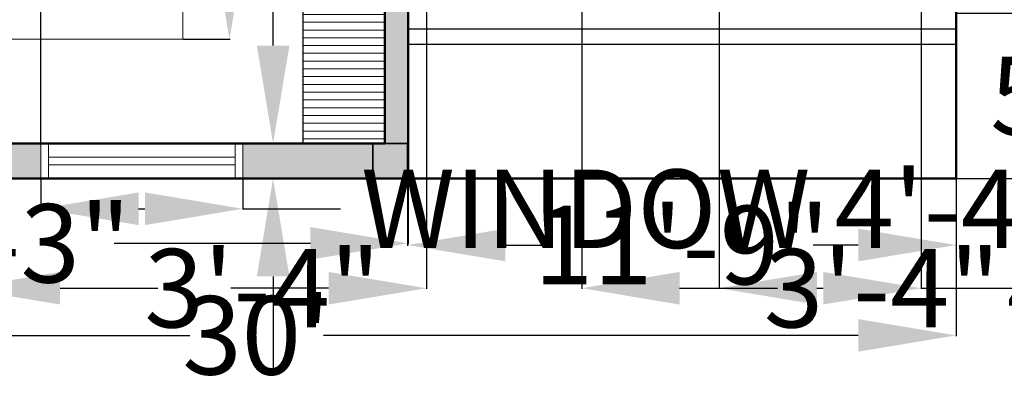
# Model space of a CAD drawing. Units: inches. Extents: x 25 to 82118, y 10 to 6494.
# Tile 3 of 9: x 40833 to 41087, y 3093 to 3189. Entities that reach past the tile are written whole.
import ezdxf

# ---------------------------------------------------------------- set-up
doc = ezdxf.new("R2010")
doc.units = ezdxf.units.IN
doc.header["$MEASUREMENT"] = 0
for name, color, linetype, lineweight in [('A-ANNO-DIMS', 2, 'Continuous', 18), ('A-FLOR-CASE', 8, 'Continuous', 25), ('A-FLOR-CASE-PATT', 9, 'Continuous', 13), ('A-FLOR-STRS', 7, 'Continuous', 25), ('A-FURN', 8, 'Continuous', 18), ('A-GLAZ', 4, 'Continuous', 18), ('A-WALL', 7, 'Continuous', 50)]:
    doc.layers.add(name, color=color, linetype=linetype, lineweight=lineweight)
doc.layers.add('A-COLS', color=30, linetype='Continuous', lineweight=35, true_color=0xf26722)
doc.layers.add('A-WALL-PATT', color=18, linetype='Continuous', lineweight=13, true_color=0x000000)
doc.styles.get("Standard").update_dxf_attribs({"font": 'arial.ttf'})
doc.dimstyles.get("Standard").update_dxf_attribs({"dimtxt": 20.18, "dimasz": 25.18, "dimexe": 0.18, "dimexo": 0.0625, "dimgap": 0.09, "dimtad": 0, "dimtih": 1, "dimtoh": 1, "dimdec": 0, "dimzin": 0, "dimdsep": 46, "dimlunit": 3, "dimtxsty": 'Standard', "dimcen": 0.09, "dimadec": 0, "dimazin": 0, "dimtfac": 1, "dimtdec": 0, "dimtofl": 0, "dimtmove": 0, "dimatfit": 3, "dimfxl": 1, "dimtolj": 1, "dimtzin": 0, "dimarcsym": 0})

# ---------------------------------------------------------------- blocks, each defined once
blk = doc.blocks.new('Bed - Queen')
for p, q in [((0, -80.00003), (0, 0)), ((0, 0), (59.99999, 0)), ((59.99999, 0), (59.99999, -80.00003)), ((7.99999, -1.2), (28.79998, -1.2)), ((7.99999, -14.4), (7.99999, -1.2)), ((28.79998, -1.2), (28.79998, -14.4)), ((31.19999, -1.2), (51.99999, -1.2)), ((31.19999, -14.4), (31.19999, -1.2)), ((51.99999, -1.2), (51.99999, -16.4)), ((0, -14.4), (44.8, -14.4)), ((59.99999, -29.6), (44.8, -14.4)), ((44.8, -14.4), (44.8, -29.6)), ((44.8, -16.8), (0, -16.8)), ((51.99999, -16.4), (46.79936, -16.4)), ((44.8, -29.6), (59.99999, -29.6)), ((59.99999, -80.00003), (0, -80.00003))]:
    blk.add_line(p, q)
blk = doc.blocks.new('*D16')
at = {"layer": 'A-ANNO-DIMS', "color": 0, "lineweight": -2, "transparency": 16777216}
for p, q in [((41074.33, 3531.88), (41191.01, 3531.88)), ((41190.83, 3506.7), (41190.83, 3350.25)), ((41190.83, 3173), (41190.83, 3329.45)), ((41074.33, 3147.82), (41191.01, 3147.82))]:
    blk.add_line(p, q, dxfattribs=at)
at = {"layer": 'A-ANNO-DIMS', "color": 0, "transparency": 16777216}
for points in [[(41186.63, 3506.7), (41195.02, 3506.7), (41190.83, 3531.88)], [(41186.63, 3173), (41195.02, 3173), (41190.83, 3147.82)]]:
    blk.add_solid(points, dxfattribs=at)
at = {"layer": 'Defpoints', "color": 0, "transparency": 16777216}
for p in [(41074.27, 3531.88), (41074.27, 3147.82), (41190.83, 3147.82)]:
    blk.add_point(p, dxfattribs=at)
at = {"layer": 'A-ANNO-DIMS', "color": 0, "transparency": 16777216, "insert": (41190.83, 3339.85), "char_height": 20.18, "attachment_point": 5}
blk.add_mtext("\\A1;32'", dxfattribs=at)
blk = doc.blocks.new('*D17')
at = {"layer": 'A-ANNO-DIMS', "color": 0, "lineweight": -2, "transparency": 16777216}
for p, q in [((41108.65, 3215.52), (41108.65, 3240.7)), ((41074.27, 3190.34), (41108.83, 3190.34)), ((41074.4, 3147.82), (41108.83, 3147.82)), ((41108.65, 3122.64), (41108.65, 3097.46))]:
    blk.add_line(p, q, dxfattribs=at)
at = {"layer": 'A-ANNO-DIMS', "color": 0, "transparency": 16777216}
for points in [[(41104.46, 3215.52), (41112.85, 3215.52), (41108.65, 3190.34)], [(41104.46, 3122.64), (41112.85, 3122.64), (41108.65, 3147.82)]]:
    blk.add_solid(points, dxfattribs=at)
at = {"layer": 'Defpoints', "color": 0, "transparency": 16777216}
for p in [(41074.21, 3190.34), (41074.33, 3147.82), (41108.65, 3147.82)]:
    blk.add_point(p, dxfattribs=at)
at = {"layer": 'A-ANNO-DIMS', "color": 0, "transparency": 16777216, "insert": (41108.65, 3169.08), "char_height": 20.18, "attachment_point": 5}
blk.add_mtext('\\A1;5\'9"', dxfattribs=at)
blk = doc.blocks.new('*D18')
at = {"layer": 'A-ANNO-DIMS', "color": 0, "lineweight": -2, "transparency": 16777216}
for p, q in [((40714.15, 3147.72), (40714.15, 3107.28)), ((41074.21, 3147.76), (41074.21, 3107.28)), ((40739.33, 3107.46), (40876.97, 3107.46)), ((41049.03, 3107.46), (40911.38, 3107.46))]:
    blk.add_line(p, q, dxfattribs=at)
at = {"layer": 'A-ANNO-DIMS', "color": 0, "transparency": 16777216}
for points in [[(40739.33, 3111.65), (40739.33, 3103.26), (40714.15, 3107.46)], [(41049.03, 3111.65), (41049.03, 3103.26), (41074.21, 3107.46)]]:
    blk.add_solid(points, dxfattribs=at)
at = {"layer": 'Defpoints', "color": 0, "transparency": 16777216}
for p in [(40714.15, 3147.79), (41074.21, 3147.82), (41074.21, 3107.46)]:
    blk.add_point(p, dxfattribs=at)
at = {"layer": 'A-ANNO-DIMS', "color": 0, "transparency": 16777216, "insert": (40894.18, 3107.46), "char_height": 20.18, "attachment_point": 5}
blk.add_mtext("\\A1;30'", dxfattribs=at)
blk = doc.blocks.new('*D19')
at = {"layer": 'A-ANNO-DIMS', "color": 0, "lineweight": -2, "transparency": 16777216}
for p, q in [((40933.06, 3147.76), (40933.06, 3130.51)), ((41074.21, 3147.76), (41074.21, 3130.51)), ((40958.24, 3130.69), (40969.83, 3130.69)), ((41049.03, 3130.69), (41037.44, 3130.69))]:
    blk.add_line(p, q, dxfattribs=at)
at = {"layer": 'A-ANNO-DIMS', "color": 0, "transparency": 16777216}
for points in [[(40958.24, 3134.89), (40958.24, 3126.49), (40933.06, 3130.69)], [(41049.03, 3134.89), (41049.03, 3126.49), (41074.21, 3130.69)]]:
    blk.add_solid(points, dxfattribs=at)
at = {"layer": 'Defpoints', "color": 0, "transparency": 16777216}
for p in [(40933.06, 3147.82), (41074.21, 3147.82), (41074.21, 3130.69)]:
    blk.add_point(p, dxfattribs=at)
at = {"layer": 'A-ANNO-DIMS', "color": 0, "transparency": 16777216, "insert": (41003.64, 3130.69), "char_height": 20.18, "attachment_point": 5}
blk.add_mtext('\\A1;11\'-9"', dxfattribs=at)
blk = doc.blocks.new('*D20')
at = {"layer": 'A-ANNO-DIMS', "color": 0, "lineweight": -2, "transparency": 16777216}
for p, q in [((40714.21, 3147.72), (40714.21, 3130.95)), ((40933.21, 3147.72), (40933.21, 3130.95)), ((40739.39, 3131.13), (40789.91, 3131.13)), ((40908.03, 3131.13), (40857.51, 3131.13))]:
    blk.add_line(p, q, dxfattribs=at)
at = {"layer": 'A-ANNO-DIMS', "color": 0, "transparency": 16777216}
for points in [[(40739.39, 3135.32), (40739.39, 3126.93), (40714.21, 3131.13)], [(40908.03, 3135.32), (40908.03, 3126.93), (40933.21, 3131.13)]]:
    blk.add_solid(points, dxfattribs=at)
at = {"layer": 'Defpoints', "color": 0, "transparency": 16777216}
for p in [(40714.21, 3147.79), (40933.21, 3147.79), (40933.21, 3131.13)]:
    blk.add_point(p, dxfattribs=at)
at = {"layer": 'A-ANNO-DIMS', "color": 0, "transparency": 16777216, "insert": (40823.71, 3131.13), "char_height": 20.18, "attachment_point": 5}
blk.add_mtext('\\A1;18\'-3"', dxfattribs=at)
blk = doc.blocks.new('WIN-48IN-9W')
for p, q in [((0, 0), (0, 9)), ((2, 0), (2, 9)), ((50, 0), (50, 9)), ((52, 0), (52, 9)), ((2, 5.5), (50, 5.5)), ((2, 3.5), (50, 3.5))]:
    blk.add_line(p, q)
blk = doc.blocks.new('COL-9X9')
h = blk.add_hatch(color=256)
h.dxf.hatch_style = 1
h.paths.add_polyline_path([(9, 9), (0, 9), (0, 0), (9, 0)])
blk.add_lwpolyline([(0, 0), (9, 0), (9, 9), (0, 9)], close=True)
blk = doc.blocks.new('*D31')
at = {"layer": 'A-ANNO-DIMS', "color": 0, "lineweight": -2, "transparency": 16777216}
for p, q in [((40838.63, 3147.76), (40838.63, 3139.84)), ((40890.63, 3147.76), (40890.63, 3139.84)), ((40863.81, 3140.02), (40865.45, 3140.02)), ((40890.63, 3140.02), (40915.81, 3140.02))]:
    blk.add_line(p, q, dxfattribs=at)
at = {"layer": 'A-ANNO-DIMS', "color": 0, "transparency": 16777216}
for points in [[(40863.81, 3144.22), (40863.81, 3135.82), (40838.63, 3140.02)], [(40865.45, 3144.22), (40865.45, 3135.82), (40890.63, 3140.02)]]:
    blk.add_solid(points, dxfattribs=at)
at = {"layer": 'Defpoints', "color": 0, "transparency": 16777216}
for p in [(40838.63, 3147.82), (40890.63, 3147.82), (40890.63, 3140.02)]:
    blk.add_point(p, dxfattribs=at)
at = {"layer": 'A-ANNO-DIMS', "color": 0, "transparency": 16777216, "insert": (41043.59, 3140.02), "char_height": 20.18, "attachment_point": 5}
blk.add_mtext('\\A1;WINDOW 4\'-4" TYP.', dxfattribs=at)
blk = doc.blocks.new('*D32')
at = {"layer": 'A-ANNO-DIMS', "color": 0, "lineweight": -2, "transparency": 16777216}
for p, q in [((40898.43, 3182), (40898.43, 3207.18)), ((40898.43, 3207.18), (40923.61, 3207.18)), ((40890.7, 3156.82), (40898.61, 3156.82)), ((40890.7, 3147.82), (40898.61, 3147.82)), ((40898.43, 3122.64), (40898.43, 3097.46))]:
    blk.add_line(p, q, dxfattribs=at)
at = {"layer": 'A-ANNO-DIMS', "color": 0, "transparency": 16777216}
for points in [[(40894.24, 3182), (40902.63, 3182), (40898.43, 3156.82)], [(40894.24, 3122.64), (40902.63, 3122.64), (40898.43, 3147.82)]]:
    blk.add_solid(points, dxfattribs=at)
at = {"layer": 'Defpoints', "color": 0, "transparency": 16777216}
for p in [(40890.63, 3156.82), (40898.43, 3156.82), (40890.63, 3147.82)]:
    blk.add_point(p, dxfattribs=at)
at = {"layer": 'A-ANNO-DIMS', "color": 0, "transparency": 16777216, "insert": (40985.21, 3207.18), "char_height": 20.18, "attachment_point": 5}
blk.add_mtext('\\A1;0\'-9" TYP.', dxfattribs=at)
blk = doc.blocks.new('*D36')
at = {"layer": 'A-ANNO-DIMS', "color": 0, "lineweight": -2, "transparency": 16777216}
for p, q in [((40887.21, 3243.62), (40887.21, 3268.8)), ((40887.21, 3268.8), (40912.39, 3268.8)), ((40875.27, 3243.62), (40887.39, 3243.62)), ((40887.21, 3208.8), (40887.21, 3218.44)), ((40875.27, 3183.62), (40887.39, 3183.62))]:
    blk.add_line(p, q, dxfattribs=at)
at = {"layer": 'A-ANNO-DIMS', "color": 0, "transparency": 16777216}
for points in [[(40883.01, 3218.44), (40891.41, 3218.44), (40887.21, 3243.62)], [(40883.01, 3208.8), (40891.41, 3208.8), (40887.21, 3183.62)]]:
    blk.add_solid(points, dxfattribs=at)
at = {"layer": 'Defpoints', "color": 0, "transparency": 16777216}
for p in [(40875.21, 3243.62), (40887.21, 3243.62), (40875.21, 3183.62)]:
    blk.add_point(p, dxfattribs=at)
at = {"layer": 'A-ANNO-DIMS', "color": 0, "transparency": 16777216, "insert": (40973.98, 3268.8), "char_height": 20.18, "attachment_point": 5}
blk.add_mtext('\\A1;5\'-0" TYP.', dxfattribs=at)
blk = doc.blocks.new('*D55')
at = {"layer": 'A-ANNO-DIMS', "color": 0, "lineweight": -2, "transparency": 16777216}
for p, q in [((40937.89, 3240.76), (40937.89, 3119.41)), ((40977.89, 3240.76), (40977.89, 3119.41)), ((40912.71, 3119.59), (40887.53, 3119.59)), ((41003.07, 3119.59), (41028.25, 3119.59))]:
    blk.add_line(p, q, dxfattribs=at)
at = {"layer": 'A-ANNO-DIMS', "color": 0, "transparency": 16777216}
for points in [[(40912.71, 3123.78), (40912.71, 3115.39), (40937.89, 3119.59)], [(41003.07, 3123.78), (41003.07, 3115.39), (40977.89, 3119.59)]]:
    blk.add_solid(points, dxfattribs=at)
at = {"layer": 'Defpoints', "color": 0, "transparency": 16777216}
for p in [(40937.89, 3240.82), (40977.89, 3240.82), (40977.89, 3119.59)]:
    blk.add_point(p, dxfattribs=at)
at = {"layer": 'A-ANNO-DIMS', "color": 0, "transparency": 16777216, "insert": (41055.16, 3119.59), "char_height": 20.18, "attachment_point": 5}
blk.add_mtext('\\A1;3\'-4"', dxfattribs=at)
blk = doc.blocks.new('*D56')
at = {"layer": 'A-ANNO-DIMS', "color": 0, "lineweight": -2, "transparency": 16777216}
for p, q in [((40778.43, 3531.76), (40778.43, 3119.41)), ((40818.43, 3531.76), (40818.43, 3119.41)), ((40753.25, 3119.59), (40728.07, 3119.59)), ((40843.61, 3119.59), (40868.79, 3119.59))]:
    blk.add_line(p, q, dxfattribs=at)
at = {"layer": 'A-ANNO-DIMS', "color": 0, "transparency": 16777216}
for points in [[(40753.25, 3123.78), (40753.25, 3115.39), (40778.43, 3119.59)], [(40843.61, 3123.78), (40843.61, 3115.39), (40818.43, 3119.59)]]:
    blk.add_solid(points, dxfattribs=at)
at = {"layer": 'Defpoints', "color": 0, "transparency": 16777216}
for p in [(40778.43, 3531.82), (40818.43, 3531.82), (40818.43, 3119.59)]:
    blk.add_point(p, dxfattribs=at)
at = {"layer": 'A-ANNO-DIMS', "color": 0, "transparency": 16777216, "insert": (40895.69, 3119.59), "char_height": 20.18, "attachment_point": 5}
blk.add_mtext('\\A1;3\'-4"', dxfattribs=at)
blk = doc.blocks.new('*D66')
at = {"layer": 'A-ANNO-DIMS', "color": 0, "lineweight": -2, "transparency": 16777216}
for p, q in [((41013.21, 3522.76), (41013.21, 3119.41)), ((41065.21, 3522.76), (41065.21, 3119.41)), ((41038.39, 3119.59), (41040.03, 3119.59)), ((41065.21, 3119.59), (41090.39, 3119.59))]:
    blk.add_line(p, q, dxfattribs=at)
at = {"layer": 'A-ANNO-DIMS', "color": 0, "transparency": 16777216}
for points in [[(41038.39, 3123.78), (41038.39, 3115.39), (41013.21, 3119.59)], [(41040.03, 3123.78), (41040.03, 3115.39), (41065.21, 3119.59)]]:
    blk.add_solid(points, dxfattribs=at)
at = {"layer": 'Defpoints', "color": 0, "transparency": 16777216}
for p in [(41013.21, 3522.82), (41065.21, 3522.82), (41065.21, 3119.59)]:
    blk.add_point(p, dxfattribs=at)
at = {"layer": 'A-ANNO-DIMS', "color": 0, "transparency": 16777216, "insert": (41117.71, 3119.59), "char_height": 20.18, "attachment_point": 5}
blk.add_mtext('\\A1;4\'-4"', dxfattribs=at)
blk = doc.blocks.new('*D67')
at = {"layer": 'A-ANNO-DIMS', "color": 0, "lineweight": -2, "transparency": 16777216}
for p, q in [((40770.03, 3572.85), (40744.85, 3572.85)), ((40795.21, 3156.88), (40795.21, 3573.03)), ((40838.63, 3156.88), (40838.63, 3573.03)), ((40863.81, 3572.85), (40888.99, 3572.85))]:
    blk.add_line(p, q, dxfattribs=at)
at = {"layer": 'A-ANNO-DIMS', "color": 0, "transparency": 16777216}
for points in [[(40770.03, 3577.05), (40770.03, 3568.66), (40795.21, 3572.85)], [(40863.81, 3577.05), (40863.81, 3568.66), (40838.63, 3572.85)]]:
    blk.add_solid(points, dxfattribs=at)
at = {"layer": 'Defpoints', "color": 0, "transparency": 16777216}
for p in [(40838.63, 3572.85), (40795.21, 3156.82), (40838.63, 3156.82)]:
    blk.add_point(p, dxfattribs=at)
at = {"layer": 'A-ANNO-DIMS', "color": 0, "transparency": 16777216, "insert": (40939.41, 3572.85), "char_height": 20.18, "attachment_point": 5}
blk.add_mtext('\\A1;3\'-7 1/2"', dxfattribs=at)
blk = doc.blocks.new('*D71')
at = {"layer": 'A-ANNO-DIMS', "color": 0, "lineweight": -2, "transparency": 16777216}
for p, q in [((41008.14, 3298.41), (41008.32, 3298.41)), ((41008.23, 3298.32), (41008.23, 3298.5)), ((41008.23, 3206.4), (41008.23, 3231.58)), ((40983.05, 3206.4), (41008.23, 3206.4))]:
    blk.add_line(p, q, dxfattribs=at)
at = {"layer": 'A-ANNO-DIMS', "color": 0, "transparency": 16777216}
blk.add_solid([(41004.03, 3231.58), (41012.42, 3231.58), (41008.23, 3256.76)], dxfattribs=at)
at = {"layer": 'Defpoints', "color": 0, "transparency": 16777216}
for p in [(41008.23, 3298.41), (41008.23, 3256.76)]:
    blk.add_point(p, dxfattribs=at)
at = {"layer": 'A-ANNO-DIMS', "color": 0, "transparency": 16777216, "insert": (40922.97, 3206.4), "char_height": 20.18, "attachment_point": 5}
blk.add_mtext('\\A1;R3\'-5 1/2"', dxfattribs=at)
blk = doc.blocks.new('*D72')
at = {"layer": 'A-ANNO-DIMS', "color": 0, "lineweight": -2, "transparency": 16777216}
for p, q in [((41008.14, 3299.19), (41008.32, 3299.19)), ((41008.23, 3299.1), (41008.23, 3299.28)), ((41008.23, 3210.55), (41008.23, 3235.73)), ((40983.05, 3210.55), (41008.23, 3210.55))]:
    blk.add_line(p, q, dxfattribs=at)
at = {"layer": 'A-ANNO-DIMS', "color": 0, "transparency": 16777216}
blk.add_solid([(41004.03, 3235.73), (41012.42, 3235.73), (41008.23, 3260.91)], dxfattribs=at)
at = {"layer": 'Defpoints', "color": 0, "transparency": 16777216}
for p in [(41008.23, 3299.19), (41008.23, 3260.91)]:
    blk.add_point(p, dxfattribs=at)
at = {"layer": 'A-ANNO-DIMS', "color": 0, "transparency": 16777216, "insert": (40922.97, 3210.55), "char_height": 20.18, "attachment_point": 5}
blk.add_mtext('\\A1;R3\'-2 1/2"', dxfattribs=at)

msp = doc.modelspace()

# ---------------------------------------------------------------- hatches: boundary and pattern name
at = {"layer": 'A-FLOR-CASE-PATT'}
h = msp.add_hatch(dxfattribs=at)
h.set_pattern_fill('ANSI31', color=256, scale=16, angle=-45, style=0)
h.paths.add_polyline_path([(40906.2, 3157.44), (40927.21, 3157.44), (40927.21, 3209.44), (40906.2, 3209.44)])
at = {"layer": 'A-WALL-PATT'}
h = msp.add_hatch(color=256, dxfattribs=at)
h.dxf.hatch_style = 1
h.paths.add_polyline_path([(40723.21, 3274), (40714.21, 3274), (40714.21, 3212.82), (40723.21, 3212.82), (40723.21, 3240.82), (40760.88, 3240.82, -0.030698), (40760.71, 3243.52), (40760.71, 3246.82), (40723.21, 3246.82)])
h.paths.add_polyline_path([(40789.21, 3246.82), (40782.73, 3246.82), (40782.73, 3243.52), (40782.73, 3240.82), (40789.21, 3240.82)])
h.paths.add_polyline_path([(40795.21, 3276.82), (40880.67, 3276.82), (40880.67, 3282.82), (40789.21, 3282.82), (40789.21, 3240.82), (40795.21, 3240.82), (40795.21, 3243.62)])
h.paths.add_polyline_path([(40795.21, 3240.82), (40789.21, 3240.82), (40789.21, 3156.82), (40723.21, 3156.82), (40723.21, 3147.82), (40838.63, 3147.82), (40838.63, 3156.82), (40795.21, 3156.82)])
h.paths.add_polyline_path([(40723.21, 3184.82), (40714.21, 3184.82), (40714.21, 3156.79), (40723.21, 3156.79), (40723.21, 3156.82)])
h.paths.add_polyline_path([(40924.06, 3156.82), (40890.63, 3156.82), (40890.63, 3147.82), (40924.06, 3147.82)])
h.paths.add_polyline_path([(40933.21, 3240.82), (40937.89, 3240.82), (40937.89, 3246.82), (40933.21, 3246.82), (40933.21, 3276.82), (40927.21, 3276.82), (40927.21, 3156.82), (40933.21, 3156.82)])
h.paths.add_polyline_path([(41000.05, 3246.82), (40977.89, 3246.82), (40977.89, 3240.82), (41000.05, 3240.82)])

# ---------------------------------------------------------------- linework, layer by layer
at = {"layer": 'A-FLOR-CASE'}
msp.add_line((40906.2, 3156.82), (40906.2, 3222.44), dxfattribs=at)
at = {"layer": 'A-FLOR-STRS'}
for p, q in [((40933.21, 3186.34), (41074.21, 3186.34)), ((40933.21, 3182.34), (41074.21, 3182.34))]:
    msp.add_line(p, q, dxfattribs=at)
at = {"layer": 'A-WALL'}
for p, q in [((41074.21, 3531.82), (41074.21, 3147.82)), ((40927.21, 3276.82), (40927.21, 3156.82)), ((40933.21, 3240.82), (40933.21, 3147.82)), ((40927.21, 3156.82), (40795.21, 3156.82)), ((41074.21, 3147.82), (40714.21, 3147.82))]:
    msp.add_line(p, q, dxfattribs=at)

# ---------------------------------------------------------------- block references
at = {"layer": 'A-COLS', "rotation": 89.99999999996236}
msp.add_blockref('COL-9X9', (40933.06, 3147.82), dxfattribs=at)
at = {"layer": 'A-FURN', "rotation": 90}
msp.add_blockref('Bed - Queen', (40795.21, 3183.62), dxfattribs=at)
at = {"layer": 'A-GLAZ'}
msp.add_blockref('WIN-48IN-9W', (40838.63, 3147.82), dxfattribs=at)

# ---------------------------------------------------------------- dimensions: what is measured, and where the dimension line sits
at = {"layer": 'A-ANNO-DIMS'}
for base, p1, p2, override, picture, middle in [((40838.63, 3572.85), (40795.21, 3156.82), (40838.63, 3156.82), {"dimdec": 1, "dimlfac": 1, "dimrnd": 0, "dimzin": 1, "dimdsep": 46, "dimlunit": 4, "dimfrac": 2}, '*D67', (40939.41, 3572.85)), ((40818.43, 3119.59), (40778.43, 3531.82), (40818.43, 3531.82), {"dimdec": 1, "dimlfac": 1, "dimrnd": 0, "dimzin": 1, "dimdsep": 46, "dimlunit": 4, "dimfrac": 2}, '*D56', (40895.69, 3119.59)), ((41065.21, 3119.59), (41013.21, 3522.82), (41065.21, 3522.82), {"dimdec": 1, "dimlfac": 1, "dimrnd": 0, "dimzin": 1, "dimdsep": 46, "dimlunit": 4, "dimfrac": 2}, '*D66', (41117.71, 3119.59)), ((40977.89, 3119.59), (40937.89, 3240.82), (40977.89, 3240.82), {"dimdec": 1, "dimlfac": 1, "dimrnd": 0, "dimzin": 1, "dimdsep": 46, "dimlunit": 4, "dimfrac": 2}, '*D55', (41055.16, 3119.59)), ((41074.21, 3107.46), (40714.15, 3147.79), (41074.21, 3147.82), {"dimclrd": 0, "dimclre": 0, "dimclrt": 0}, '*D18', (40894.18, 3107.46)), ((40933.21, 3131.13), (40714.21, 3147.79), (40933.21, 3147.79), {"dimclrd": 0, "dimclre": 0, "dimclrt": 0}, '*D20', (40823.71, 3131.13)), ((41074.21, 3130.69), (40933.06, 3147.82), (41074.21, 3147.82), {"dimclrd": 0, "dimclre": 0, "dimclrt": 0}, '*D19', (41003.64, 3130.69))]:
    dim = msp.add_linear_dim(base=base, p1=p1, p2=p2, dimstyle='Standard', override=override, dxfattribs=at)
    dim.commit()
    dim.dimension.update_dxf_attribs({"geometry": picture, "text_midpoint": middle})
dim = msp.add_linear_dim(base=(41190.83, 3147.82), p1=(41074.27, 3531.88), p2=(41074.27, 3147.82), angle=90, dimstyle='Standard', override={"dimclrd": 0, "dimclre": 0, "dimclrt": 0}, dxfattribs=at)
dim.commit()
dim.dimension.update_dxf_attribs({"geometry": '*D16', "text_midpoint": (41190.83, 3339.85)})
for center, mpoint, picture, middle in [((41008.23, 3299.19), (41008.23, 3260.91), '*D72', (40922.97, 3210.55)), ((41008.2264, 3298.4101), (41008.226, 3256.7602), '*D71', (40922.9662, 3206.4002))]:
    dim = msp.add_radius_dim(center=center, mpoint=mpoint, dimstyle='Standard', override={"dimdec": 1, "dimlfac": 1, "dimrnd": 0, "dimzin": 1, "dimdsep": 46, "dimlunit": 4, "dimfrac": 2}, dxfattribs=at)
    dim.commit()
    dim.dimension.update_dxf_attribs({"geometry": picture, "text_midpoint": middle})
for base, p1, p2, text, override, picture, middle in [((40887.21, 3243.62), (40875.21, 3183.62), (40875.21, 3243.62), '<> TYP.', {"dimdec": 1, "dimlfac": 1, "dimrnd": 0, "dimzin": 1, "dimdsep": 46, "dimlunit": 4, "dimfrac": 2}, '*D36', (40973.98, 3268.8)), ((41108.65, 3147.82), (41074.21, 3190.34), (41074.33, 3147.82), '5\'9"', {"dimclrd": 0, "dimclre": 0, "dimclrt": 0}, '*D17', (41108.65, 3169.08)), ((40898.43, 3156.82), (40890.63, 3147.82), (40890.63, 3156.82), '<> TYP.', {"dimdec": 1, "dimlfac": 1, "dimrnd": 0, "dimzin": 1, "dimdsep": 46, "dimlunit": 4, "dimfrac": 2}, '*D32', (40985.21, 3207.18))]:
    dim = msp.add_linear_dim(base=base, p1=p1, p2=p2, angle=90, text=text, dimstyle='Standard', override=override, dxfattribs=at)
    dim.commit()
    dim.dimension.update_dxf_attribs({"geometry": picture, "text_midpoint": middle})
dim = msp.add_linear_dim(base=(40890.63, 3140.02), p1=(40838.63, 3147.82), p2=(40890.63, 3147.82), text='WINDOW <> TYP.', dimstyle='Standard', override={"dimdec": 1, "dimlfac": 1, "dimrnd": 0, "dimzin": 1, "dimdsep": 46, "dimlunit": 4, "dimfrac": 2}, dxfattribs=at)
dim.commit()
dim.dimension.update_dxf_attribs({"geometry": '*D31', "text_midpoint": (41043.59, 3140.02)})

doc.saveas('drawing.dxf')
